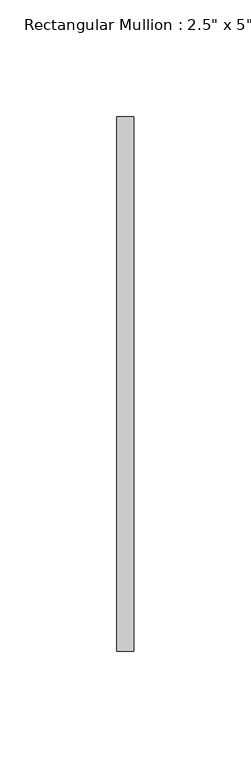
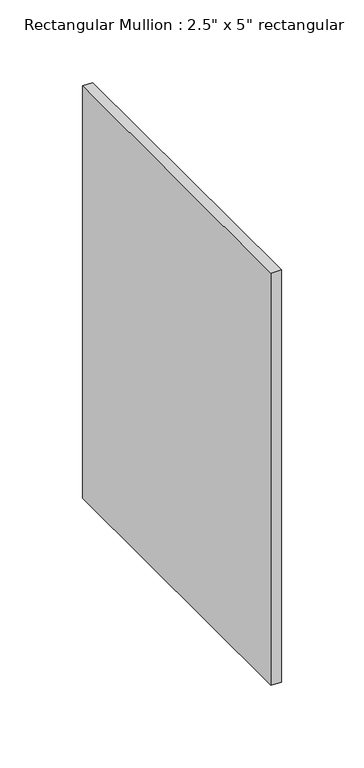
"""IFC4 building model written with IfcOpenShell, lengths in millimetres: member geometry."""

from ifc_helpers import new_model, si_unit, frame, origin, place, context, project, spatial, polyline, outline, extrude, source, transform, mapped, element, save


def member_579a4f36(model_context):
    return source(origin(), model_context, "Body", "SweptSolid", [
        extrude(outline(polyline([(0.0, 114.3), (0.0, -114.3), (-7.239, -114.3), (-7.239, 114.3), (0.0, 114.3)])), frame((0.0, 0.0, -304.8), z_axis=(0.0, 0.0, 1.0), x_axis=(1.0, 0.0, 0.0)), (0.0, 0.0, 1.0), 304.8),
    ])


if __name__ == "__main__":
    model = new_model("IFC4")
    model_context = context("Model", 3, world=origin())
    ifc_project = project(units=[si_unit("LENGTHUNIT", "METRE", prefix="MILLI")], contexts=[model_context])
    site = spatial("IfcSite", under=ifc_project)
    building = spatial("IfcBuilding", under=site)
    placement = place(None, origin())
    member_shape = member_579a4f36(model_context)
    element("IfcMember", 1, ObjectType="Rectangular Mullion : 2.5\" x 5\" rectangular", at=placement, inside=building, context=model_context, shape_type="MappedRepresentation", body=[
        mapped(member_shape, transform((0.0, 0.0, 0.0), x_axis=(1.0, 0.0, 0.0), y_axis=(0.0, 1.0, 0.0), z_axis=(0.0, 0.0, 1.0))),
    ])
    save(model, "model.ifc")

# Revit data of these elements
# Type "Rectangular Mullion : 2.5\" x 5\" rectangular"
#   built-in parameter 1007304 = 0.75 (stored number, unit not read)
#   built-in parameter 1007301 = 0.011875 (stored number, unit not read)
#   built-in parameter 1007300 = 0.011875 (stored number, unit not read)
# Element 1 (IfcMember, "Rectangular Mullion : 2.5\" x 5\" rectangular")
#   Materials on its faces: "WINDOW GLASS MATERIAL"
# Materials
#   "WINDOW GLASS MATERIAL": class "Generic", colour RGB 120 120 120, transparency 0, Cost = 0
